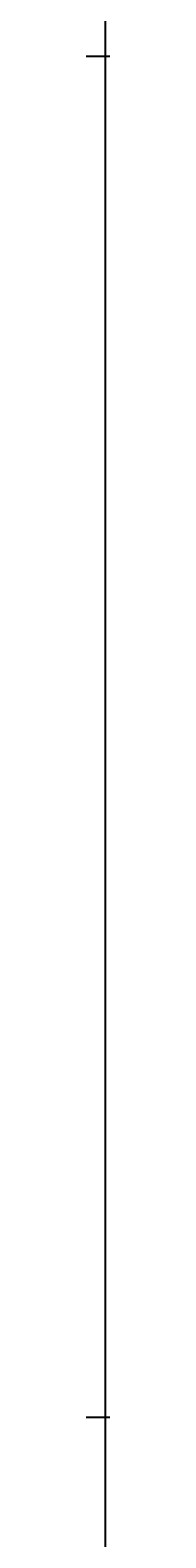
# Model space of a CAD drawing. Units: inches. Extents: x 35362 to 73946, y 43607 to 67532.
# Tile 22 of 134: x 48371 to 48372, y 46091 to 46564. Entities that reach past the tile are written whole.
import ezdxf

# ---------------------------------------------------------------- set-up
doc = ezdxf.new("R2010")
doc.units = ezdxf.units.IN
doc.header["$MEASUREMENT"] = 0
doc.layers.add('A-ANNO-DIMS', color=2, linetype='Continuous', lineweight=18)
doc.styles.get("Standard").update_dxf_attribs({"font": 'arial.ttf'})
doc.dimstyles.get("Standard").update_dxf_attribs({"dimtxt": 0.18, "dimasz": 0.18, "dimexe": 0.18, "dimexo": 0.0625, "dimgap": 0.09, "dimtad": 0, "dimtih": 1, "dimtoh": 1, "dimdec": 4, "dimzin": 0, "dimdsep": 46, "dimtxsty": 'Standard', "dimcen": 0.09, "dimadec": 0, "dimazin": 0, "dimtfac": 1, "dimtdec": 4, "dimtofl": 0, "dimtmove": 0, "dimatfit": 3, "dimfxl": 1, "dimtolj": 1, "dimtzin": 0, "dimarcsym": 0})

# ---------------------------------------------------------------- blocks, each defined once
blk = doc.blocks.new('*D5')
at = {"layer": 'A-ANNO-DIMS', "color": 0, "lineweight": -2, "transparency": 16777216}
for p, q in [((37121.95, 46919.32), (37121.95, 43606.68)), ((69871.5, 45449.83), (69871.5, 43606.68)), ((37122.13, 43606.86), (53496.29, 43606.86)), ((69871.32, 43606.86), (53497.15, 43606.86))]:
    blk.add_line(p, q, dxfattribs=at)
at = {"layer": 'A-ANNO-DIMS', "color": 0, "transparency": 16777216}
for points in [[(37122.13, 43606.89), (37122.13, 43606.83), (37121.95, 43606.86)], [(69871.32, 43606.89), (69871.32, 43606.83), (69871.5, 43606.86)]]:
    blk.add_solid(points, dxfattribs=at)
at = {"layer": 'Defpoints', "color": 0, "transparency": 16777216}
for p in [(37121.95, 46919.38), (69871.5, 45449.89), (69871.5, 43606.86)]:
    blk.add_point(p, dxfattribs=at)
at = {"layer": 'A-ANNO-DIMS', "color": 0, "transparency": 16777216, "insert": (53496.72, 43606.86), "char_height": 0.18, "attachment_point": 5}
blk.add_mtext('\\A1;32750', dxfattribs=at)
blk = doc.blocks.new('*D11')
at = {"layer": 'A-ANNO-DIMS', "color": 0, "lineweight": -2, "transparency": 16777216}
for p, q in [((47978.66, 56028.77), (47978.66, 43606.68)), ((53109.76, 56028.77), (53109.76, 43606.68)), ((47978.84, 43606.86), (50543.87, 43606.86)), ((53109.58, 43606.86), (50544.55, 43606.86))]:
    blk.add_line(p, q, dxfattribs=at)
at = {"layer": 'A-ANNO-DIMS', "color": 0, "transparency": 16777216}
for points in [[(47978.84, 43606.89), (47978.84, 43606.83), (47978.66, 43606.86)], [(53109.58, 43606.89), (53109.58, 43606.83), (53109.76, 43606.86)]]:
    blk.add_solid(points, dxfattribs=at)
at = {"layer": 'Defpoints', "color": 0, "transparency": 16777216}
for p in [(47978.66, 56028.84), (53109.76, 56028.84), (53109.76, 43606.86)]:
    blk.add_point(p, dxfattribs=at)
at = {"layer": 'A-ANNO-DIMS', "color": 0, "transparency": 16777216, "insert": (50544.21, 43606.86), "char_height": 0.18, "attachment_point": 5}
blk.add_mtext('\\A1;5131', dxfattribs=at)
blk = doc.blocks.new('*D27')
at = {"layer": 'A-ANNO-DIMS', "color": 0, "lineweight": -2, "transparency": 16777216}
for p, q in [((47978.66, 56028.77), (47978.66, 43606.68)), ((48373.49, 53428.96), (48373.49, 43606.68)), ((47978.84, 43606.86), (48175.68, 43606.86)), ((48373.31, 43606.86), (48176.47, 43606.86))]:
    blk.add_line(p, q, dxfattribs=at)
at = {"layer": 'A-ANNO-DIMS', "color": 0, "transparency": 16777216}
for points in [[(47978.84, 43606.89), (47978.84, 43606.83), (47978.66, 43606.86)], [(48373.31, 43606.89), (48373.31, 43606.83), (48373.49, 43606.86)]]:
    blk.add_solid(points, dxfattribs=at)
at = {"layer": 'Defpoints', "color": 0, "transparency": 16777216}
for p in [(47978.66, 56028.84), (48373.49, 53429.02), (48373.49, 43606.86)]:
    blk.add_point(p, dxfattribs=at)
at = {"layer": 'A-ANNO-DIMS', "color": 0, "transparency": 16777216, "insert": (48176.08, 43606.86), "char_height": 0.18, "attachment_point": 5}
blk.add_mtext('\\A1;394.8', dxfattribs=at)
blk = doc.blocks.new('*D67')
at = {"layer": 'A-ANNO-DIMS', "color": 0, "lineweight": -2, "transparency": 16777216}
for p, q in [((56873.54, 53351.53), (35361.77, 53351.53)), ((35361.95, 53351.35), (35361.95, 49400.89)), ((35361.95, 45450.07), (35361.95, 49400.53)), ((53793.58, 45449.89), (35361.77, 45449.89))]:
    blk.add_line(p, q, dxfattribs=at)
at = {"layer": 'A-ANNO-DIMS', "color": 0, "transparency": 16777216}
for points in [[(35361.92, 53351.35), (35361.98, 53351.35), (35361.95, 53351.53)], [(35361.92, 45450.07), (35361.98, 45450.07), (35361.95, 45449.89)]]:
    blk.add_solid(points, dxfattribs=at)
at = {"layer": 'Defpoints', "color": 0, "transparency": 16777216}
for p in [(35361.95, 53351.53), (56873.6, 53351.53), (53793.64, 45449.89)]:
    blk.add_point(p, dxfattribs=at)
at = {"layer": 'A-ANNO-DIMS', "color": 0, "transparency": 16777216, "insert": (35361.95, 49400.71), "char_height": 0.18, "attachment_point": 5}
blk.add_mtext('\\A1;7901.6', dxfattribs=at)
blk = doc.blocks.new('*D76')
at = {"layer": 'A-ANNO-DIMS', "color": 0, "lineweight": -2, "transparency": 16777216}
for p, q in [((54052.84, 46555.29), (35361.77, 46555.29)), ((35361.95, 46555.11), (35361.95, 46342.27)), ((35361.95, 46129.06), (35361.95, 46341.9)), ((53793.58, 46128.88), (35361.77, 46128.88))]:
    blk.add_line(p, q, dxfattribs=at)
at = {"layer": 'A-ANNO-DIMS', "color": 0, "transparency": 16777216}
for points in [[(35361.92, 46555.11), (35361.98, 46555.11), (35361.95, 46555.29)], [(35361.92, 46129.06), (35361.98, 46129.06), (35361.95, 46128.88)]]:
    blk.add_solid(points, dxfattribs=at)
at = {"layer": 'Defpoints', "color": 0, "transparency": 16777216}
for p in [(35361.95, 46555.29), (54052.9, 46555.29), (53793.64, 46128.88)]:
    blk.add_point(p, dxfattribs=at)
at = {"layer": 'A-ANNO-DIMS', "color": 0, "transparency": 16777216, "insert": (35361.95, 46342.09), "char_height": 0.18, "attachment_point": 5}
blk.add_mtext('\\A1;426.4', dxfattribs=at)
blk = doc.blocks.new('*D90')
at = {"layer": 'A-ANNO-DIMS', "color": 0, "lineweight": -2, "transparency": 16777216}
for p, q in [((53707.72, 47291.29), (35361.77, 47291.29)), ((35361.95, 47291.11), (35361.95, 46710.26)), ((35361.95, 46129.06), (35361.95, 46709.9)), ((53793.58, 46128.88), (35361.77, 46128.88))]:
    blk.add_line(p, q, dxfattribs=at)
at = {"layer": 'A-ANNO-DIMS', "color": 0, "transparency": 16777216}
for points in [[(35361.92, 47291.11), (35361.98, 47291.11), (35361.95, 47291.29)], [(35361.92, 46129.06), (35361.98, 46129.06), (35361.95, 46128.88)]]:
    blk.add_solid(points, dxfattribs=at)
at = {"layer": 'Defpoints', "color": 0, "transparency": 16777216}
for p in [(53707.78, 47291.29), (35361.95, 46128.88), (53793.64, 46128.88)]:
    blk.add_point(p, dxfattribs=at)
at = {"layer": 'A-ANNO-DIMS', "color": 0, "transparency": 16777216, "insert": (35361.95, 46710.08), "char_height": 0.18, "attachment_point": 5}
blk.add_mtext('\\A1;1162.4', dxfattribs=at)

msp = doc.modelspace()

# ---------------------------------------------------------------- dimensions: what is measured, and where the dimension line sits
at = {"layer": 'A-ANNO-DIMS'}
for base, p1, p2, override, picture, middle in [((53109.76, 43606.859), (47978.665, 56028.836), (53109.76, 56028.836), {"dimdec": 0, "dimlfac": 1, "dimrnd": 0, "dimzin": 0, "dimdsep": 46, "dimlunit": 2}, '*D11', (50544.212, 43606.859)), ((48373.492, 43606.859), (47978.665, 56028.836), (48373.492, 53429.019), {"dimdec": 1, "dimlfac": 1, "dimrnd": 0, "dimzin": 0, "dimdsep": 46, "dimlunit": 2}, '*D27', (48176.078, 43606.859)), ((69871.496, 43606.859), (37121.949, 46919.381), (69871.496, 45449.894), {"dimdec": 0, "dimlfac": 1, "dimrnd": 0, "dimzin": 0, "dimdsep": 46, "dimlunit": 2}, '*D5', (53496.723, 43606.859))]:
    dim = msp.add_linear_dim(base=base, p1=p1, p2=p2, dimstyle='Standard', override=override, dxfattribs=at)
    dim.commit()
    dim.dimension.update_dxf_attribs({"geometry": picture, "text_midpoint": middle})
for base, p1, p2, picture, middle in [((35361.949, 53351.529), (53793.638, 45449.894), (56873.602, 53351.529), '*D67', (35361.949, 49400.712)), ((35361.949, 46128.878), (53707.781, 47291.285), (53793.638, 46128.878), '*D90', (35361.949, 46710.081)), ((35361.949, 46555.293), (53793.638, 46128.878), (54052.899, 46555.293), '*D76', (35361.949, 46342.086))]:
    dim = msp.add_linear_dim(base=base, p1=p1, p2=p2, angle=90, dimstyle='Standard', override={"dimdec": 1, "dimlfac": 1, "dimrnd": 0, "dimzin": 0, "dimdsep": 46, "dimlunit": 2}, dxfattribs=at)
    dim.commit()
    dim.dimension.update_dxf_attribs({"geometry": picture, "text_midpoint": middle})

doc.saveas('drawing.dxf')
